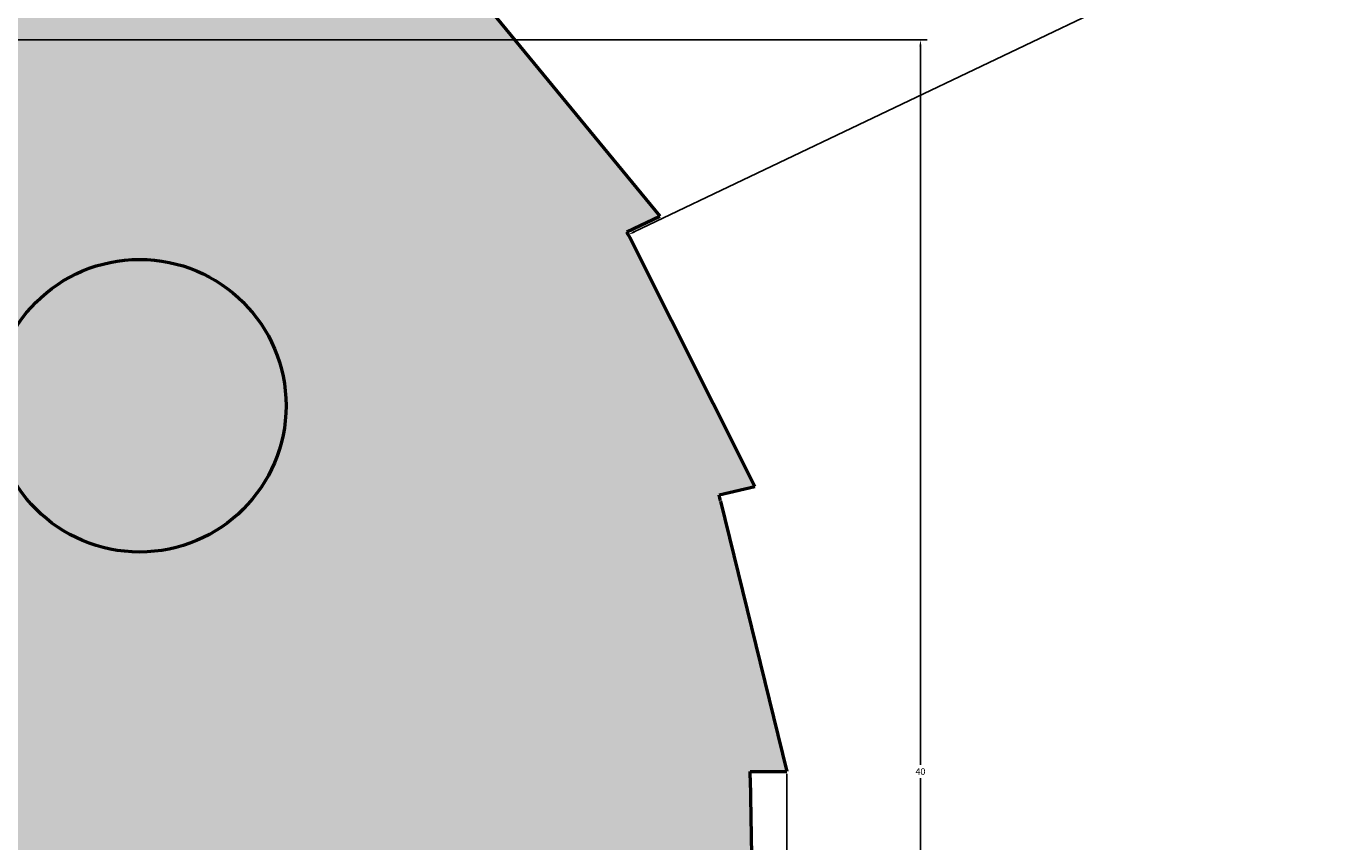
# Model space of a CAD drawing. Units: millimetres. Extents: x 2943.6 to 3032.7, y 1562 to 1639.7.
# Tile 8 of 9: x 2996.7 to 3032.7, y 1598.9 to 1621.2. Entities that reach past the tile are written whole.
import ezdxf

# ---------------------------------------------------------------- set-up
doc = ezdxf.new("R2010")
doc.units = ezdxf.units.MM
doc.layers.add('M-DIMS', color=2, linetype='Continuous', lineweight=18)
doc.layers.add('M-OUTL', color=7, linetype='Continuous', lineweight=50)
doc.layers.add('M-HATC', color=7, linetype='Continuous', lineweight=18, true_color=0xffffff)
doc.styles.get("Standard").update_dxf_attribs({"font": 'arial.ttf'})
doc.dimstyles.get("Standard").update_dxf_attribs({"dimtxt": 0.18, "dimasz": 0.18, "dimexe": 0.18, "dimexo": 0.0625, "dimgap": 0.09, "dimtad": 0, "dimtih": 1, "dimtoh": 1, "dimdec": 4, "dimzin": 0, "dimdsep": 46, "dimtxsty": 'Standard', "dimcen": 0.09, "dimadec": 0, "dimazin": 0, "dimtfac": 1, "dimtdec": 4, "dimtofl": 0, "dimtmove": 0, "dimatfit": 3, "dimfxl": 1, "dimtolj": 1, "dimtzin": 0, "dimarcsym": 0})

# ---------------------------------------------------------------- blocks, each defined once
blk = doc.blocks.new('*U1')
blk.add_circle((0, 0), 4)
blk = doc.blocks.new('*U2')
at = {"layer": 'M-OUTL', "color": 0, "linetype": 'ByBlock', "lineweight": -2, "transparency": 16777216, "rotation": 300}
blk.add_blockref('*U1', (2999.79, 1610.848), dxfattribs=at)
blk = doc.blocks.new('*D3')
at = {"layer": 'Defpoints', "color": 0, "transparency": 16777216}
for p in [(2947.469, 1600.848), (3017.469, 1600.848), (3017.469, 1562.198)]:
    blk.add_point(p, dxfattribs=at)
at = {"layer": 'M-DIMS', "color": 0, "lineweight": -2, "transparency": 16777216}
for p, q in [((2947.469, 1600.786), (2947.469, 1562.018)), ((3017.469, 1600.786), (3017.469, 1562.018)), ((2947.649, 1562.198), (2982.251, 1562.198)), ((3017.289, 1562.198), (2982.687, 1562.198))]:
    blk.add_line(p, q, dxfattribs=at)
at = {"layer": 'M-DIMS', "color": 0, "transparency": 16777216}
for points in [[(2947.649, 1562.228), (2947.649, 1562.168), (2947.469, 1562.198)], [(3017.289, 1562.228), (3017.289, 1562.168), (3017.469, 1562.198)]]:
    blk.add_solid(points, dxfattribs=at)
at = {"layer": 'M-DIMS', "color": 0, "transparency": 16777216, "insert": (2982.469, 1562.198), "char_height": 0.18, "attachment_point": 5}
blk.add_mtext('\\A1;70', dxfattribs=at)
blk = doc.blocks.new('*D5')
at = {"layer": 'Defpoints', "color": 0, "transparency": 16777216}
for p in [(2986.469, 1620.848), (3021.119, 1620.848), (2986.469, 1580.848)]:
    blk.add_point(p, dxfattribs=at)
at = {"layer": 'M-DIMS', "color": 0, "lineweight": -2, "transparency": 16777216}
for p, q in [((2986.532, 1620.848), (3021.299, 1620.848)), ((3021.119, 1620.668), (3021.119, 1601.03)), ((3021.119, 1581.028), (3021.119, 1600.666)), ((2986.532, 1580.848), (3021.299, 1580.848))]:
    blk.add_line(p, q, dxfattribs=at)
at = {"layer": 'M-DIMS', "color": 0, "transparency": 16777216}
for points in [[(3021.089, 1620.668), (3021.149, 1620.668), (3021.119, 1620.848)], [(3021.089, 1581.028), (3021.149, 1581.028), (3021.119, 1580.848)]]:
    blk.add_solid(points, dxfattribs=at)
at = {"layer": 'M-DIMS', "color": 0, "transparency": 16777216, "insert": (3021.119, 1600.848), "char_height": 0.18, "attachment_point": 5}
blk.add_mtext('\\A1;40', dxfattribs=at)
blk = doc.blocks.new('*D10')
at = {"layer": 'Defpoints', "color": 0, "transparency": 16777216}
for p in [(3013.14, 1615.522), (2982.469, 1600.848)]:
    blk.add_point(p, dxfattribs=at)
at = {"layer": 'M-DIMS', "color": 0, "lineweight": -2, "transparency": 16777216}
for p, q in [((3031.542, 1624.326), (3013.302, 1615.6)), ((3031.722, 1624.326), (3031.542, 1624.326)), ((2982.379, 1600.848), (2982.559, 1600.848)), ((2982.469, 1600.758), (2982.469, 1600.938))]:
    blk.add_line(p, q, dxfattribs=at)
at = {"layer": 'M-DIMS', "color": 0, "transparency": 16777216}
blk.add_solid([(3013.289, 1615.627), (3013.315, 1615.573), (3013.14, 1615.522)], dxfattribs=at)
at = {"layer": 'M-DIMS', "color": 0, "transparency": 16777216, "insert": (3032.292, 1624.326), "char_height": 0.18, "attachment_point": 5}
blk.add_mtext('\\A1;28X R34', dxfattribs=at)

msp = doc.modelspace()

# ---------------------------------------------------------------- hatches: boundary and pattern name
at = {"layer": 'M-HATC'}
h = msp.add_hatch(color=256, dxfattribs=at)
h.set_gradient(color1=(0, 0, 255), color2=(255, 255, 0), tint=1, name='INVCURVED')
h.paths.add_polyline_path([(2949.361, 1608.583, 0.001279), (2949.322, 1608.414), (2948.347, 1608.637), (2948.473, 1600.848), (2947.469, 1600.848), (2949.283, 1593.452, 0.001279), (2949.322, 1593.283), (2948.347, 1593.06), (2951.761, 1586.253, 0.001279), (2951.836, 1586.096), (2950.935, 1585.662), (2955.779, 1579.786, 0.001279), (2955.887, 1579.65), (2955.105, 1579.026), (2961.135, 1574.375, 0.001279), (2961.271, 1574.266), (2960.647, 1573.484), (2967.561, 1570.291, 0.001279), (2967.717, 1570.215), (2967.283, 1569.314), (2974.734, 1567.74, 0.001279), (2974.904, 1567.701), (2974.681, 1566.726), (2982.295, 1566.849, 0.001279), (2982.469, 1566.848), (2982.469, 1565.848), (2989.865, 1567.662, 0.001279), (2990.035, 1567.701), (2990.258, 1566.726), (2997.064, 1570.14, 0.001279), (2997.221, 1570.215), (2997.655, 1569.314), (3003.532, 1574.158, 0.001279), (3003.668, 1574.266), (3004.291, 1573.484), (3008.943, 1579.514, 0.001279), (3009.052, 1579.65), (3009.833, 1579.026), (3013.026, 1585.94, 0.001279), (3013.102, 1586.096), (3014.003, 1585.662), (3015.578, 1593.113, 0.001279), (3015.617, 1593.283), (3016.592, 1593.06), (3016.469, 1600.674, 0.001279), (3016.469, 1600.848), (3017.469, 1600.848), (3015.655, 1608.244, 0.001279), (3015.617, 1608.414), (3016.592, 1608.637), (3013.177, 1615.443, 0.001279), (3013.102, 1615.6), (3014.003, 1616.034), (3009.16, 1621.911, 0.001279), (3009.052, 1622.047), (3009.833, 1622.67), (3003.804, 1627.322, 0.001279), (3003.668, 1627.431), (3004.291, 1628.212), (2997.378, 1631.405, 0.001279), (2997.221, 1631.481), (2997.655, 1632.382), (2990.204, 1633.957, 0.001279), (2990.035, 1633.996), (2990.258, 1634.971), (2982.469, 1634.845), (2982.469, 1635.848), (2975.073, 1634.034, 0.001279), (2974.904, 1633.996), (2974.681, 1634.971), (2967.874, 1631.556, 0.001279), (2967.717, 1631.481), (2967.283, 1632.382), (2961.407, 1627.539, 0.001279), (2961.271, 1627.431), (2960.647, 1628.212), (2955.996, 1622.183, 0.001279), (2955.887, 1622.047), (2955.105, 1622.67), (2951.912, 1615.757, 0.001279), (2951.836, 1615.6), (2950.935, 1616.034)])
h.paths.add_polyline_path([(2969.149, 1610.848, -1), (2961.149, 1610.848, -1)], flags=16)
h.paths.add_polyline_path([(2969.149, 1590.848, -1), (2961.149, 1590.848, -1)], flags=16)
h.paths.add_polyline_path([(2992.469, 1600.848, -1), (2972.469, 1600.848, -1)], flags=16)
h.paths.add_polyline_path([(2978.469, 1620.848, -1), (2986.469, 1620.848, -1)], flags=16)
h.paths.add_polyline_path([(2981.469, 1605.236), (2981.469, 1606.848), (2983.469, 1606.848), (2983.469, 1605.236, -8.887482)], flags=0)
h.paths.add_polyline_path([(2986.469, 1580.848, -1), (2978.469, 1580.848, -1)], flags=16)
h.paths.add_polyline_path([(3003.79, 1610.848, -1), (2995.79, 1610.848, -1)], flags=16)
h.paths.add_polyline_path([(3003.79, 1590.848, -1), (2995.79, 1590.848, -1)], flags=16)
h = msp.add_hatch(color=256, dxfattribs=at)
h.paths.add_polyline_path([(2978.469, 1620.848, 1), (2986.469, 1620.848, 1)])
h.paths.add_polyline_path([(2995.79, 1610.848, 1), (3003.79, 1610.848, 1)])
h.paths.add_polyline_path([(3003.79, 1590.848, 1), (2995.79, 1590.848, 1)])
h.paths.add_polyline_path([(2986.469, 1580.848, 1), (2978.469, 1580.848, 1)])
h.paths.add_polyline_path([(2969.149, 1590.848, 1), (2961.149, 1590.848, 1)])
h.paths.add_polyline_path([(2961.149, 1610.848, 1), (2969.149, 1610.848, 1)])

# ---------------------------------------------------------------- linework, layer by layer
at = {"layer": 'M-OUTL'}
for p, q in [((3009.16, 1621.911), (3014.003, 1616.034)), ((3013.102, 1615.6), (3014.003, 1616.034)), ((3013.177, 1615.443), (3016.592, 1608.637)), ((3015.617, 1608.414), (3016.592, 1608.637)), ((3015.655, 1608.244), (3017.469, 1600.848)), ((3016.469, 1600.848), (3017.469, 1600.848)), ((3016.469, 1600.674), (3016.592, 1593.06))]:
    msp.add_line(p, q, dxfattribs=at)
for start, end in [(25.4212, 25.7143), (12.564, 12.8571), (359.7069, 360)]:
    msp.add_arc((2982.469, 1600.848), 34, start, end, dxfattribs=at)

# ---------------------------------------------------------------- block references
msp.add_blockref('*U2', (0, 0), dxfattribs=at)

# ---------------------------------------------------------------- dimensions: what is measured, and where the dimension line sits
at = {"layer": 'M-DIMS'}
dim = msp.add_radius_dim(center=(2982.469, 1600.848), mpoint=(3013.14, 1615.522), text='28X <>', dimstyle='Standard', override={"dimdec": 0, "dimlfac": 1, "dimrnd": 0, "dimzin": 0, "dimdsep": 46, "dimlunit": 2}, dxfattribs=at)
dim.commit()
dim.dimension.update_dxf_attribs({"geometry": '*D10', "text_midpoint": (3032.292, 1624.326), "dimtype": 164})
dim = msp.add_linear_dim(base=(3021.119, 1620.848), p1=(2986.469, 1580.848), p2=(2986.469, 1620.848), angle=90, dimstyle='Standard', override={"dimdec": 0, "dimlfac": 1, "dimrnd": 0, "dimzin": 0, "dimdsep": 46, "dimlunit": 2}, dxfattribs=at)
dim.commit()
dim.dimension.update_dxf_attribs({"geometry": '*D5', "text_midpoint": (3021.119, 1600.848)})
dim = msp.add_linear_dim(base=(3017.469, 1562.198), p1=(2947.469, 1600.848), p2=(3017.469, 1600.848), dimstyle='Standard', override={"dimdec": 0, "dimlfac": 1, "dimrnd": 0, "dimzin": 0, "dimdsep": 46, "dimlunit": 2}, dxfattribs=at)
dim.commit()
dim.dimension.update_dxf_attribs({"geometry": '*D3', "text_midpoint": (2982.469, 1562.198)})

doc.saveas('drawing.dxf')
